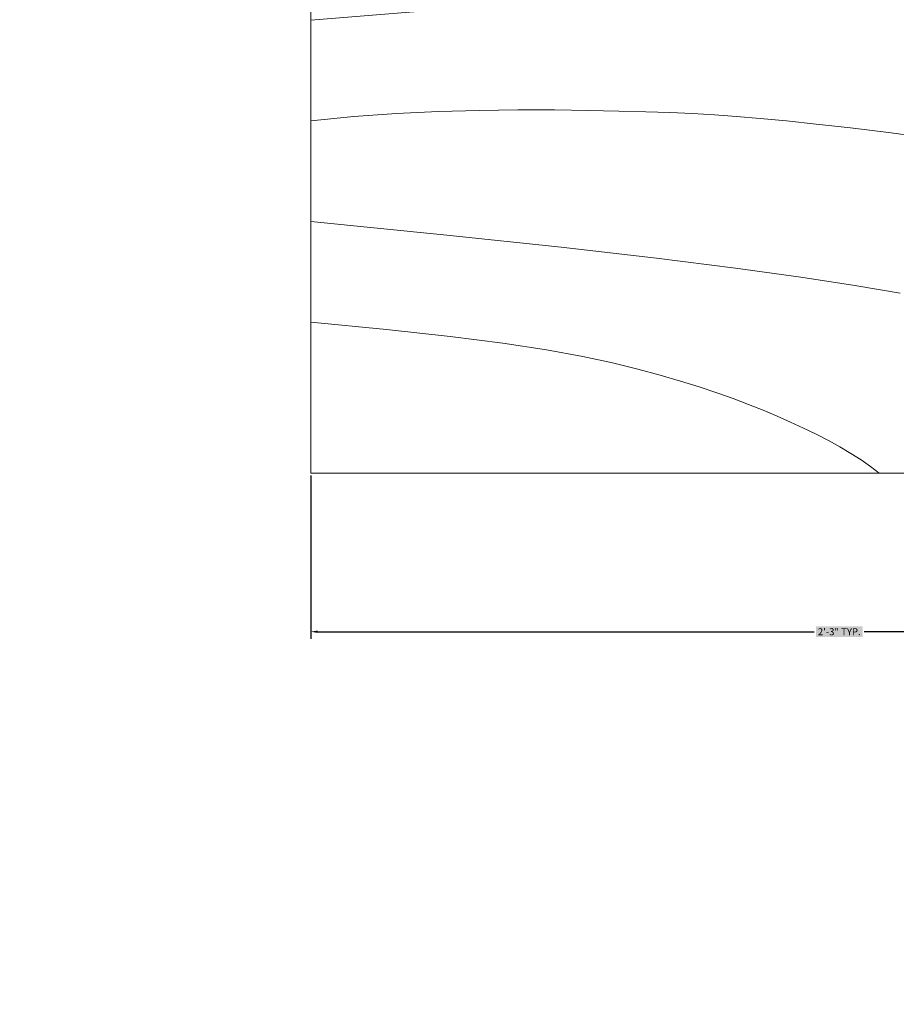
# Model space of a CAD drawing. Units: inches. Extents: x -128 to 854, y -395 to 398.
# Tile 38 of 61: x 270 to 292, y 145 to 170. Entities that reach past the tile are written whole.
import ezdxf

# ---------------------------------------------------------------- set-up
doc = ezdxf.new("R2010")
doc.units = ezdxf.units.IN
doc.header["$MEASUREMENT"] = 0
doc.layers.add('A-ANNO-DIMS', color=2, linetype='Continuous', lineweight=18)
doc.layers.add('A-FURN', color=8, linetype='Continuous', lineweight=18)
doc.styles.get("Standard").update_dxf_attribs({"font": 'arial.ttf'})
doc.dimstyles.get("Standard").update_dxf_attribs({"dimtxt": 0.18, "dimasz": 0.18, "dimexe": 0.18, "dimexo": 0.0625, "dimgap": 0.09, "dimtad": 0, "dimtih": 1, "dimtoh": 1, "dimdec": 1, "dimzin": 0, "dimdsep": 46, "dimlunit": 4, "dimtxsty": 'Standard', "dimcen": 0.09, "dimclrd": 1, "dimclre": 2, "dimclrt": 6, "dimadec": 0, "dimazin": 0, "dimtfac": 1, "dimtdec": 1, "dimtofl": 0, "dimtmove": 0, "dimatfit": 3, "dimfxl": 1, "dimtfill": 2, "dimtfillclr": 3, "dimtolj": 1, "dimtzin": 0, "dimarcsym": 0})

# ---------------------------------------------------------------- blocks, each defined once
blk = doc.blocks.new('Table - Square Woodgrain 42 x 42 in.')
blk.add_line((0, -42), (42, -42))
for points in [[(0, -42), (0, 0), (42, 0), (42, -42)], [(0, -24), (3.9243, -23.6805), (7.4766, -23.4138), (10.6891, -23.1954), (13.5943, -23.0205), (16.2247, -22.8847), (18.6125, -22.7832), (20.7903, -22.7116), (22.7903, -22.6651), (24.6563, -22.642), (26.4764, -22.6507), (28.35, -22.7024), (30.3766, -22.8084), (32.6555, -22.98), (35.2861, -23.2283), (38.3678, -23.5645), (42, -24)], [(25.0009, -28.742), (23.0612, -28.4707), (21.4439, -28.2716), (20.0786, -28.1215), (18.8998, -28.0002), (17.8609, -27.9014), (16.9206, -27.8219), (16.0371, -27.7588), (15.1691, -27.709), (14.2748, -27.6693), (13.3128, -27.6368), (12.2415, -27.6083), (11.0295, -27.5824), (9.6867, -27.5643), (8.233, -27.5608), (6.6884, -27.5787), (5.0728, -27.6248), (3.4062, -27.7058), (1.7086, -27.8286), (0, -28)], [(0, -32), (5.4026, -32.5358), (9.9494, -33.019), (13.7424, -33.4553), (16.8834, -33.8505), (19.4743, -34.2106), (21.6171, -34.5413), (23.4136, -34.8486)], [(0, -36), (3.0098, -36.2857), (5.5354, -36.5643), (7.6368, -36.8359), (9.374, -37.1009), (10.807, -37.3597), (11.9957, -37.6126), (13.0002, -37.8599), (13.8804, -38.102), (14.6874, -38.3393), (15.4365, -38.5729), (16.1338, -38.8041), (16.7858, -39.0341), (17.3987, -39.264), (17.9787, -39.4952), (18.5322, -39.7288), (19.0655, -39.9662), (19.5832, -40.2081), (20.0842, -40.4544), (20.5657, -40.7046), (21.0249, -40.9581), (21.459, -41.2144), (21.8653, -41.4731), (22.2409, -41.7335), (22.5831, -41.9951)]]:
    blk.add_lwpolyline(points)
blk = doc.blocks.new('*D55')
at = {"layer": 'A-ANNO-DIMS', "color": 0, "lineweight": -2, "transparency": 16777216}
for p, q in [((304.81, 186.741), (221.092, 186.741)), ((221.272, 181.741), (221.272, 131.873)), ((221.272, 77.741), (221.272, 127.608)), ((304.81, 72.741), (221.092, 72.741))]:
    blk.add_line(p, q, dxfattribs=at)
at = {"layer": 'A-ANNO-DIMS', "color": 0, "transparency": 16777216}
for points in [[(220.439, 181.741), (222.105, 181.741), (221.272, 186.741)], [(220.439, 77.741), (222.105, 77.741), (221.272, 72.741)]]:
    blk.add_solid(points, dxfattribs=at)
at = {"layer": 'Defpoints', "color": 0, "transparency": 16777216}
for p in [(221.272, 186.741), (304.873, 186.741), (304.873, 72.741)]:
    blk.add_point(p, dxfattribs=at)
at = {"layer": 'A-ANNO-DIMS', "color": 0, "transparency": 16777216, "insert": (221.272, 129.741), "char_height": 4, "attachment_point": 5, "bg_fill": 1, "box_fill_scale": 1.25, "bg_fill_color": 3, "bg_fill_transparency": 0}
blk.add_mtext('\\A1;9\'-6"', dxfattribs=at)
blk = doc.blocks.new('*D88')
at = {"layer": 'A-ANNO-DIMS', "color": 2, "lineweight": -2, "transparency": 16777216}
for p, q in [((277.284, 158.766), (277.284, 154.585)), ((304.372, 158.766), (304.372, 154.585))]:
    blk.add_line(p, q, dxfattribs=at)
at = {"layer": 'A-ANNO-DIMS', "color": 1, "lineweight": -2, "transparency": 16777216}
for p, q in [((277.464, 154.765), (290.188, 154.765)), ((304.192, 154.765), (291.468, 154.765))]:
    blk.add_line(p, q, dxfattribs=at)
at = {"layer": 'A-ANNO-DIMS', "color": 1, "transparency": 16777216}
for points in [[(277.464, 154.795), (277.464, 154.735), (277.284, 154.765)], [(304.192, 154.795), (304.192, 154.735), (304.372, 154.765)]]:
    blk.add_solid(points, dxfattribs=at)
at = {"layer": 'Defpoints', "color": 0, "transparency": 16777216}
for p in [(277.284, 158.828), (304.372, 158.828), (304.372, 154.765)]:
    blk.add_point(p, dxfattribs=at)
at = {"layer": 'A-ANNO-DIMS', "color": 6, "transparency": 16777216, "insert": (290.828, 154.765), "char_height": 0.18, "attachment_point": 5, "bg_fill": 1, "box_fill_scale": 1.25, "bg_fill_color": 3, "bg_fill_transparency": 0}
blk.add_mtext('\\A1;2\'-3" TYP.', dxfattribs=at)

msp = doc.modelspace()

# ---------------------------------------------------------------- block references
at = {"layer": 'A-FURN', "xscale": 0.6449685946951323, "yscale": 0.6449685946951323, "zscale": 0.6449685946951323}
msp.add_blockref('Table - Square Woodgrain 42 x 42 in.', (277.284, 185.917), dxfattribs=at)

# ---------------------------------------------------------------- dimensions: what is measured, and where the dimension line sits
at = {"layer": 'A-ANNO-DIMS'}
dim = msp.add_linear_dim(base=(221.272, 186.741), p1=(304.873, 72.741), p2=(304.873, 186.741), angle=90, dimstyle='Standard', override={"dimtxt": 4, "dimasz": 5, "dimclrd": 0, "dimclre": 0, "dimclrt": 0}, dxfattribs=at)
dim.commit()
dim.dimension.update_dxf_attribs({"geometry": '*D55', "text_midpoint": (221.272, 129.741)})
dim = msp.add_linear_dim(base=(304.372, 154.765), p1=(277.284, 158.828), p2=(304.372, 158.828), text='<> TYP.', dimstyle='Standard', override={"dimdec": 1, "dimlfac": 1, "dimrnd": 0, "dimzin": 1, "dimdsep": 46, "dimlunit": 4, "dimfrac": 2}, dxfattribs=at)
dim.commit()
dim.dimension.update_dxf_attribs({"geometry": '*D88', "text_midpoint": (290.828, 154.765)})

doc.saveas('drawing.dxf')
